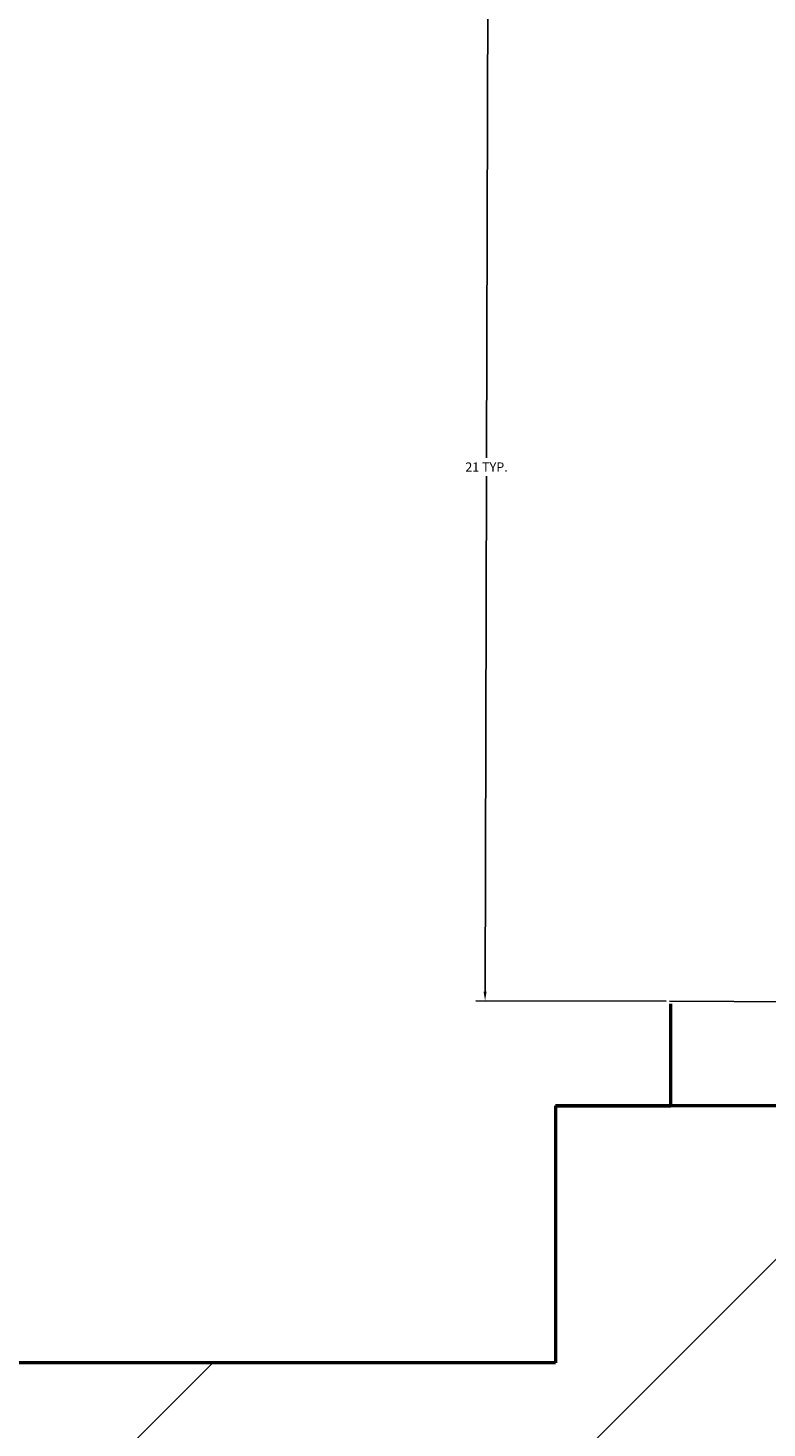
# Model space of a CAD drawing. Units: inches. Extents: x 1901 to 2863, y 888 to 2433.
# Tile 80 of 91: x 2645 to 2659, y 2009 to 2037. Entities that reach past the tile are written whole.
import ezdxf

# ---------------------------------------------------------------- set-up
doc = ezdxf.new("R2010")
doc.units = ezdxf.units.IN
for name, color, linetype, lineweight in [('A-ANNO-DIMS', 2, 'Continuous', 18), ('A-DOOR', 4, 'Continuous', 25), ('A-WALL', 7, 'Continuous', 50), ('A-WALL-PATT', 8, 'Continuous', 13)]:
    doc.layers.add(name, color=color, linetype=linetype, lineweight=lineweight)
doc.styles.get("Standard").update_dxf_attribs({"font": 'arial.ttf'})
doc.dimstyles.get("Standard").update_dxf_attribs({"dimtxt": 0.18, "dimasz": 0.18, "dimexe": 0.18, "dimexo": 0.0625, "dimgap": 0.09, "dimtad": 0, "dimtih": 1, "dimtoh": 1, "dimdec": 4, "dimzin": 0, "dimdsep": 46, "dimtxsty": 'Standard', "dimcen": 0.09, "dimadec": 0, "dimazin": 0, "dimtfac": 1, "dimtdec": 4, "dimtofl": 0, "dimtmove": 0, "dimatfit": 3, "dimfxl": 1, "dimtolj": 1, "dimtzin": 0, "dimarcsym": 0})

# ---------------------------------------------------------------- blocks, each defined once
blk = doc.blocks.new('DOOR-20B')
blk.add_line((0.002, -0.016), (0.002, 23.984))
blk.add_arc((0.002, 3.902), 20.082, 348.7487, 90)
blk = doc.blocks.new('*D40')
at = {"layer": 'A-ANNO-DIMS', "color": 0, "lineweight": -2, "transparency": 16777216}
for p, q in [((2657.145, 2038.567), (2653.428, 2038.577)), ((2653.607, 2038.397), (2653.58, 2028.323)), ((2653.551, 2017.888), (2653.579, 2027.962)), ((2657.088, 2017.698), (2653.371, 2017.708))]:
    blk.add_line(p, q, dxfattribs=at)
at = {"layer": 'A-ANNO-DIMS', "color": 0, "transparency": 16777216}
for points in [[(2653.577, 2038.397), (2653.637, 2038.397), (2653.608, 2038.577)], [(2653.521, 2017.888), (2653.581, 2017.888), (2653.551, 2017.708)]]:
    blk.add_solid(points, dxfattribs=at)
at = {"layer": 'Defpoints', "color": 0, "transparency": 16777216}
for p in [(2653.608, 2038.577), (2657.208, 2038.567), (2657.151, 2017.698)]:
    blk.add_point(p, dxfattribs=at)
at = {"layer": 'A-ANNO-DIMS', "color": 0, "transparency": 16777216, "insert": (2653.579, 2028.142), "char_height": 0.18, "attachment_point": 5}
blk.add_mtext('\\A1;21 TYP.', dxfattribs=at)

msp = doc.modelspace()

# ---------------------------------------------------------------- hatches: boundary and pattern name
at = {"layer": 'A-WALL-PATT'}
h = msp.add_hatch(dxfattribs=at)
h.set_pattern_fill('ANSI32', color=256)
h.paths.add_polyline_path([(2192.501, 2274.134), (2141.264, 2274.134), (2141.264, 2269.634), (2192.501, 2269.634)])
h.paths.add_polyline_path([(2259.926, 2274.134), (2216.501, 2274.134), (2216.501, 2269.634), (2255.426, 2269.634), (2255.426, 2214.634), (2250.809, 2214.634), (2250.809, 2210.134), (2259.926, 2210.134), (2259.926, 2215.134), (2271.756, 2215.134), (2271.756, 2217.384), (2271.756, 2219.634), (2259.926, 2219.634)])
h.paths.add_polyline_path([(2171.426, 2269.634), (2166.926, 2269.634), (2166.926, 2219.634), (2121.238, 2219.634), (2121.238, 2215.134), (2166.926, 2215.134), (2166.926, 2083.134), (2161.807, 2083.134), (2161.807, 2078.634), (2171.426, 2078.634), (2176.996, 2078.634), (2176.996, 2080.884), (2176.996, 2083.134), (2171.426, 2083.134), (2171.426, 2210.134), (2230.912, 2210.134), (2230.912, 2212.384), (2230.912, 2214.634), (2171.426, 2214.634)])
h.paths.add_polyline_path([(2117.264, 2274.134), (2089.426, 2274.134), (2089.426, 2219.634), (2081.136, 2219.634), (2081.136, 2215.134), (2089.426, 2215.134), (2098.004, 2215.134), (2098.004, 2217.384), (2098.004, 2219.634), (2093.926, 2219.634), (2093.926, 2269.634), (2117.264, 2269.634), (2117.264, 2271.884)])
h.paths.add_polyline_path([(2343.426, 2219.634), (2329.295, 2219.634), (2329.295, 2215.134), (2338.926, 2215.134), (2338.926, 2184.739), (2343.426, 2184.739)])
h.paths.add_polyline_path([(2338.926, 2083.134), (2329.295, 2083.134), (2208.966, 2083.134), (2208.966, 2078.634), (2338.926, 2078.634)])
h.paths.add_polyline_path([(2343.426, 2136.739), (2338.926, 2136.739), (2338.926, 1872.634), (2343.426, 1872.634)])
h.paths.add_polyline_path([(2343.426, 1863.634), (2397.68, 1863.634), (2397.68, 1821.634), (2384.138, 1821.634), (2384.138, 1812.634), (2418.33, 1812.634), (2418.33, 1817.134), (2418.33, 1821.634), (2406.68, 1821.634), (2406.68, 1863.634), (2459.499, 1863.634), (2459.499, 1821.634), (2447.138, 1821.634), (2447.138, 1812.634), (2459.499, 1812.634), (2468.499, 1812.634), (2468.499, 1872.634), (2394.426, 1872.634), (2334.426, 1872.634), (2334.426, 1812.634), (2343.426, 1812.634), (2353.251, 1812.634), (2353.251, 1821.634), (2343.426, 1821.634)])
h.paths.add_polyline_path([(2510.014, 1872.634), (2468.499, 1872.634), (2468.499, 1868.134), (2510.014, 1868.134)])
h.paths.add_polyline_path([(2514.009, 1817.134), (2468.499, 1817.134), (2468.499, 1812.634), (2482.114, 1812.634), (2482.114, 1800.606), (2486.614, 1800.606), (2486.614, 1812.634), (2514.009, 1812.634)])
h.paths.add_polyline_path([(2299.247, 1814.884), (2299.247, 1817.134), (2295.926, 1817.134), (2295.926, 1854.169), (2293.676, 1854.169), (2291.426, 1854.169), (2291.426, 1817.134), (2266.109, 1817.134), (2266.109, 1812.634), (2299.247, 1812.634)])
h.paths.add_polyline_path([(2218.109, 1817.134), (2206.46, 1817.134), (2171.426, 1817.134), (2171.426, 1949.134), (2190.1, 1949.134), (2190.1, 1953.634), (2163.468, 1953.634), (2163.468, 1949.134), (2166.926, 1949.134), (2166.926, 1817.134), (2114.297, 1817.134), (2114.297, 1812.634), (2218.109, 1812.634)])
h.paths.add_polyline_path([(2029.426, 1970.922), (2024.926, 1970.922), (2024.926, 1912.717), (2029.426, 1912.717)])
h.paths.add_polyline_path([(2132.297, 1953.634), (2113.926, 1953.634), (2113.926, 1975.888), (2111.676, 1975.888), (2109.426, 1975.888), (2109.426, 1953.634), (2029.426, 1953.634), (2029.426, 1949.134), (2132.297, 1949.134)])
h.paths.add_polyline_path([(2029.426, 1853.606), (2029.31, 1853.606), (2029.31, 1853.606), (2029.426, 1853.606), (2029.426, 1864.717), (2024.926, 1864.717), (2024.926, 1812.634), (2066.297, 1812.634), (2066.297, 1814.884), (2066.297, 1817.134), (2029.426, 1817.134)])
h.paths.add_polyline_path([(2122.926, 2010.088), (2120.676, 2010.088), (2118.426, 2010.088), (2118.426, 2006.134), (2029.426, 2006.134), (2029.426, 2001.634), (2109.426, 2001.634), (2109.426, 1998.041), (2113.926, 1998.041), (2113.926, 2001.634), (2122.926, 2001.634)])
h.paths.add_polyline_path([(2029.426, 2031.376), (2024.926, 2031.376), (2024.926, 1994.922), (2027.176, 1994.922), (2029.426, 1994.922)])
h.paths.add_polyline_path([(2029.426, 2136.739), (2024.926, 2136.739), (2024.926, 2067.376), (2027.176, 2067.376), (2029.426, 2067.376)])
h.paths.add_polyline_path([(2125.618, 2083.134), (2029.426, 2083.134), (2029.426, 2078.634), (2118.426, 2078.634), (2118.426, 2030.715), (2122.926, 2030.715), (2122.926, 2078.634), (2125.618, 2078.634)])
h.paths.add_polyline_path([(2029.426, 2215.134), (2040.468, 2215.134), (2040.468, 2217.384), (2040.468, 2219.634), (2024.926, 2219.634), (2024.926, 2184.739), (2029.426, 2184.739), (2029.426, 2187.778)])
h.paths.add_polyline_path([(2686.426, 2274.134), (2659.284, 2274.134), (2659.284, 2269.634), (2681.926, 2269.634), (2681.926, 2219.634), (2676.816, 2219.634), (2676.816, 2215.134), (2681.926, 2215.134), (2697.011, 2215.134), (2697.011, 2217.384), (2697.011, 2219.634), (2686.426, 2219.634)])
h.paths.add_polyline_path([(2609.926, 2269.634), (2635.284, 2269.634), (2635.284, 2274.134), (2571.431, 2274.134), (2571.431, 2269.634), (2605.426, 2269.634), (2605.426, 2214.634), (2549.098, 2214.634), (2549.098, 2210.134), (2605.426, 2210.134), (2605.426, 2083.134), (2601.014, 2083.134), (2601.014, 2080.884), (2601.014, 2078.634), (2609.926, 2078.634), (2616.162, 2078.634), (2616.162, 2080.884), (2616.162, 2083.134), (2609.926, 2083.134), (2609.926, 2215.134), (2651.465, 2215.134), (2651.465, 2217.384), (2651.465, 2219.634), (2609.926, 2219.634)])
h.paths.add_polyline_path([(2521.426, 2269.634), (2547.431, 2269.634), (2547.431, 2271.884), (2547.431, 2274.134), (2516.926, 2274.134), (2516.926, 2219.634), (2506.41, 2219.634), (2506.41, 2215.134), (2516.926, 2215.134), (2516.926, 2210.134), (2525.402, 2210.134), (2525.402, 2212.384), (2525.402, 2214.634), (2521.426, 2214.634)])
h.paths.add_polyline_path([(2456.011, 2219.634), (2439.426, 2219.634), (2439.426, 2187.888), (2443.926, 2187.888), (2443.926, 2215.134), (2456.011, 2215.134)])
h.paths.add_polyline_path([(2752.926, 2219.634), (2739.485, 2219.634), (2739.485, 2215.134), (2748.426, 2215.134), (2748.426, 2187.888), (2752.926, 2187.888)])
h.paths.add_polyline_path([(2752.926, 2139.888), (2748.426, 2139.888), (2748.426, 2083.134), (2648.416, 2083.134), (2648.416, 2078.634), (2654.926, 2078.634), (2654.926, 2039.437), (2659.426, 2039.437), (2659.426, 2078.634), (2748.426, 2078.634), (2748.426, 2063.429), (2752.926, 2063.429)])
h.paths.add_polyline_path([(2752.926, 2010.634), (2659.426, 2010.634), (2659.426, 2015.652), (2654.926, 2015.652), (2654.926, 2010.634), (2605.426, 2010.634), (2605.426, 1920.967), (2609.926, 1920.967), (2609.926, 2006.134), (2748.426, 2006.134), (2748.426, 1982.466), (2752.926, 1982.466)])
h.paths.add_polyline_path([(2752.926, 2027.429), (2748.426, 2027.429), (2748.426, 2010.634), (2752.926, 2010.634)])
h.paths.add_polyline_path([(2748.426, 1886.134), (2609.926, 1886.134), (2609.926, 1889.719), (2605.426, 1889.719), (2605.426, 1861.262), (2609.926, 1861.262), (2609.926, 1881.634), (2748.426, 1881.634)])
h.paths.add_polyline_path([(2456.855, 2228.831), (2498.401, 2228.831), (2498.401, 2247.488), (2456.855, 2247.488)], flags=9)
h.paths.add_polyline_path([(2038.602, 2237.418), (2080.174, 2237.418), (2080.174, 2256.075), (2038.602, 2256.075)], flags=9)
h.paths.add_polyline_path([(2292.009, 1062.394), (2539.932, 1062.394), (2539.932, 1099.487), (2292.009, 1099.487)], flags=9)
h.paths.add_polyline_path([(2424.91, 1832.253), (2448.513, 1832.253), (2448.513, 1846.678), (2424.91, 1846.678)], flags=25)
h.paths.add_polyline_path([(2359.076, 1832.253), (2382.678, 1832.253), (2382.678, 1846.678), (2359.076, 1846.678)], flags=25)
h.paths.add_polyline_path([(2352.899, 1684.802), (2367.543, 1684.802), (2367.543, 1697.167), (2352.899, 1697.167)], flags=9)
h.paths.add_polyline_path([(2079.288, 1755.826), (2169.024, 1755.826), (2169.024, 1774.372), (2079.288, 1774.372)], flags=9)
h.paths.add_polyline_path([(2404.09, 1373.857), (2404.09, 1463.593), (2385.544, 1463.593), (2385.544, 1373.857)], flags=9)
h.paths.add_polyline_path([(2268.091, 2236.371), (2309.636, 2236.371), (2309.636, 2255.028), (2268.091, 2255.028)], flags=9)
h.paths.add_polyline_path([(2575.96, 1700.951), (2665.696, 1700.951), (2665.696, 1719.498), (2575.96, 1719.498)], flags=9)
h.paths.add_polyline_path([(2302.962, 1878.474), (2329.524, 1878.474), (2329.524, 1888.777), (2302.962, 1888.777)], flags=9)
h.paths.add_polyline_path([(2097.415, 2240.576), (2126.573, 2240.576), (2126.573, 2259.233), (2097.415, 2259.233)], flags=9)
h.paths.add_polyline_path([(2208.725, 2246.124), (2237.882, 2246.124), (2237.882, 2264.781), (2208.725, 2264.781)], flags=9)
h.paths.add_polyline_path([(2038.147, 1925.958), (2076.987, 1925.958), (2076.987, 1944.615), (2038.147, 1944.615)], flags=9)
h.paths.add_polyline_path([(2239.144, 1926.672), (2288.465, 1926.672), (2288.465, 1945.329), (2239.144, 1945.329)], flags=9)
h.paths.add_polyline_path([(2175.429, 2007.33), (2212.356, 2007.33), (2212.356, 2025.987), (2175.429, 2025.987)], flags=9)
h.paths.add_polyline_path([(2225.034, 2091.794), (2263.875, 2091.794), (2263.875, 2110.451), (2225.034, 2110.451)], flags=9)
h.paths.add_polyline_path([(2035.398, 2098.478), (2074.238, 2098.478), (2074.238, 2117.135), (2035.398, 2117.135)], flags=9)
h.paths.add_polyline_path([(2050.102, 2029.209), (2083.26, 2029.209), (2083.26, 2047.866), (2050.102, 2047.866)], flags=9)
h.paths.add_polyline_path([(2069.677, 1956.719), (2098.835, 1956.719), (2098.835, 1975.376), (2069.677, 1975.376)], flags=25)
h.paths.add_polyline_path([(2328.62, 1753.336), (2361.663, 1753.336), (2361.663, 1771.993), (2328.62, 1771.993)], flags=9)
h.paths.add_polyline_path([(2395.162, 2060.888), (2395.162, 2140.654), (2378.676, 2140.654), (2378.676, 2060.888)], flags=9)
h.paths.add_polyline_path([(2463.728, 2059.02), (2492.886, 2059.02), (2492.886, 2077.677), (2463.728, 2077.677)], flags=9)
h.paths.add_polyline_path([(2458.027, 2181.536), (2496.868, 2181.536), (2496.868, 2200.194), (2458.027, 2200.194)], flags=9)
h.paths.add_polyline_path([(2527.577, 2243.074), (2556.735, 2243.074), (2556.735, 2261.731), (2527.577, 2261.731)], flags=9)
h.paths.add_polyline_path([(2694.461, 2232.767), (2736.033, 2232.767), (2736.033, 2251.425), (2694.461, 2251.425)], flags=9)
h.paths.add_polyline_path([(2637.821, 2249.225), (2666.979, 2249.225), (2666.979, 2267.882), (2637.821, 2267.882)], flags=9)
h.paths.add_polyline_path([(2623.687, 2183.541), (2662.528, 2183.541), (2662.528, 2202.199), (2623.687, 2202.199)], flags=9)
h.paths.add_polyline_path([(2691.965, 2021.5), (2725.124, 2021.5), (2725.124, 2040.157), (2691.965, 2040.157)], flags=9)
h.paths.add_polyline_path([(2621.043, 1975.912), (2662.335, 1975.912), (2662.335, 1994.569), (2621.043, 1994.569)], flags=25)
h.paths.add_polyline_path([(2479.032, 1927.62), (2519.844, 1927.62), (2519.844, 1946.277), (2479.032, 1946.277)], flags=9)
h.paths.add_polyline_path([(2670.941, 1849.076), (2716.005, 1849.076), (2716.005, 1867.734), (2670.941, 1867.734)], flags=9)
h.paths.add_polyline_path([(2523.613, 1782.956), (2550.175, 1782.956), (2550.175, 1793.26), (2523.613, 1793.26)], flags=9)
h.paths.add_polyline_path([(2450.841, 1207.331), (2492.386, 1207.331), (2492.386, 1225.989), (2450.841, 1225.989)], flags=9)
h.paths.add_polyline_path([(2527.751, 1203.841), (2556.908, 1203.841), (2556.908, 1222.499), (2527.751, 1222.499)], flags=9)
h.paths.add_polyline_path([(2639.111, 1207.2), (2668.268, 1207.2), (2668.268, 1225.857), (2639.111, 1225.857)], flags=9)
h.paths.add_polyline_path([(2692.594, 1218.965), (2734.167, 1218.965), (2734.167, 1237.623), (2692.594, 1237.623)], flags=9)
h.paths.add_polyline_path([(2669.266, 1366.329), (2708.106, 1366.329), (2708.106, 1384.987), (2669.266, 1384.987)], flags=9)
h.paths.add_polyline_path([(2463.313, 1358.031), (2502.153, 1358.031), (2502.153, 1376.688), (2463.313, 1376.688)], flags=9)
h.paths.add_polyline_path([(2494.725, 1449.963), (2531.652, 1449.963), (2531.652, 1468.62), (2494.725, 1468.62)], flags=9)
h.paths.add_polyline_path([(2675.565, 1422.157), (2708.724, 1422.157), (2708.724, 1440.815), (2675.565, 1440.815)], flags=9)
h.paths.add_polyline_path([(2685.634, 1493.891), (2714.792, 1493.891), (2714.792, 1512.548), (2685.634, 1512.548)], flags=9)
h.paths.add_polyline_path([(2686.805, 1529.913), (2725.645, 1529.913), (2725.645, 1548.57), (2686.805, 1548.57)], flags=9)
h.paths.add_polyline_path([(2503.651, 1537.991), (2552.972, 1537.991), (2552.972, 1556.648), (2503.651, 1556.648)], flags=9)
h.paths.add_polyline_path([(2291.713, 1643.504), (2318.275, 1643.504), (2318.275, 1653.807), (2291.713, 1653.807)], flags=9)
h.paths.add_polyline_path([(2450.626, 1610.52), (2477.189, 1610.52), (2477.189, 1620.824), (2450.626, 1620.824)], flags=9)
h.paths.add_polyline_path([(2359.985, 1551.814), (2422.253, 1551.814), (2422.253, 1562.117), (2359.985, 1562.117)], flags=9)
h.paths.add_polyline_path([(2280.106, 1249.006), (2321.651, 1249.006), (2321.651, 1267.663), (2280.106, 1267.663)], flags=9)
h.paths.add_polyline_path([(2164.057, 1274.232), (2193.215, 1274.232), (2193.215, 1292.889), (2164.057, 1292.889)], flags=9)
h.paths.add_polyline_path([(2118.21, 1277.694), (2151.252, 1277.694), (2151.252, 1296.351), (2118.21, 1296.351)], flags=9)
h.paths.add_polyline_path([(2031.946, 1268.529), (2073.519, 1268.529), (2073.519, 1287.187), (2031.946, 1287.187)], flags=9)
h.paths.add_polyline_path([(2050.199, 1409.079), (2089.04, 1409.079), (2089.04, 1427.736), (2050.199, 1427.736)], flags=9)
h.paths.add_polyline_path([(2243.743, 1421.032), (2282.584, 1421.032), (2282.584, 1439.689), (2243.743, 1439.689)], flags=9)
h.paths.add_polyline_path([(2190.746, 1509.769), (2231.558, 1509.769), (2231.558, 1528.426), (2190.746, 1528.426)], flags=9)
h.paths.add_polyline_path([(2058.392, 1475.415), (2091.55, 1475.415), (2091.55, 1494.073), (2058.392, 1494.073)], flags=9)
h.paths.add_polyline_path([(2062.447, 1553.09), (2091.605, 1553.09), (2091.605, 1571.747), (2062.447, 1571.747)], flags=9)
h.paths.add_polyline_path([(2219.524, 1590.365), (2266.147, 1590.365), (2266.147, 1609.022), (2219.524, 1609.022)], flags=9)
h.paths.add_polyline_path([(2041.072, 1584.188), (2079.912, 1584.188), (2079.912, 1602.845), (2041.072, 1602.845)], flags=9)

# ---------------------------------------------------------------- linework, layer by layer
at = {"layer": 'A-WALL'}
for p, q in [((2657.176, 2015.652), (2657.176, 2017.652)), ((2659.426, 2015.652), (2654.926, 2015.652)), ((2654.926, 2015.652), (2657.176, 2015.652)), ((2654.926, 2015.652), (2654.926, 2010.634)), ((2654.926, 2010.634), (2605.426, 2010.634))]:
    msp.add_line(p, q, dxfattribs=at)

# ---------------------------------------------------------------- block references
at = {"layer": 'A-DOOR', "extrusion": (0, 0, -1), "zscale": -1, "rotation": 90.1553947244059}
msp.add_blockref('DOOR-20B', (-2657.167, 2017.696), dxfattribs=at)

# ---------------------------------------------------------------- dimensions: what is measured, and where the dimension line sits
at = {"layer": 'A-ANNO-DIMS'}
dim = msp.add_linear_dim(base=(2653.608, 2038.577), p1=(2657.151, 2017.698), p2=(2657.208, 2038.567), angle=89.8446, text='<> TYP.', dimstyle='Standard', override={"dimdec": 0, "dimlfac": 1, "dimrnd": 0, "dimzin": 0, "dimdsep": 46, "dimlunit": 2}, dxfattribs=at)
dim.commit()
dim.dimension.update_dxf_attribs({"geometry": '*D40', "text_midpoint": (2653.579, 2028.142)})

doc.saveas('drawing.dxf')
